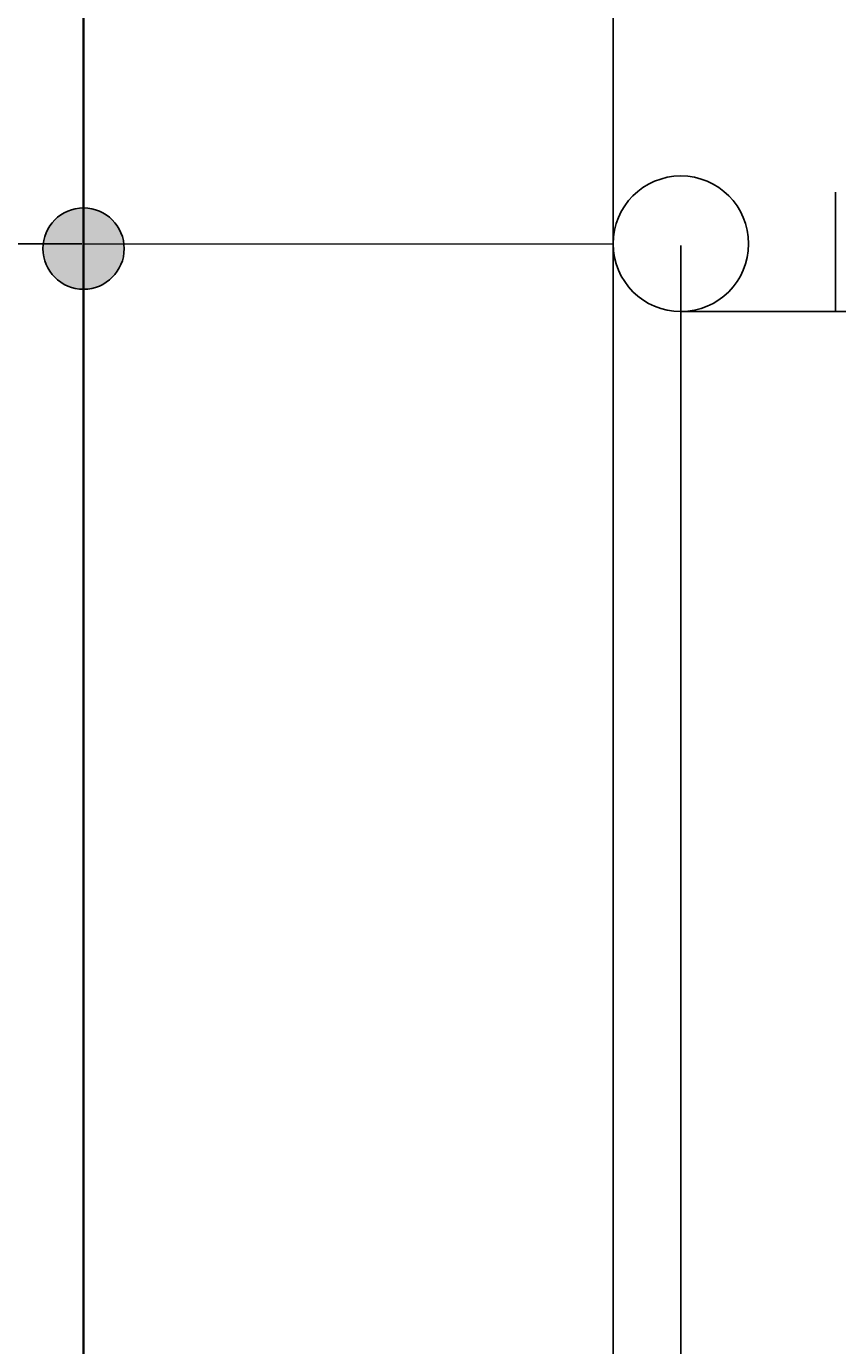
# Model space of a CAD drawing. Units: inches. Extents: x 738 to 1068, y 378 to 757.
# Tile 34 of 41: x 779 to 809, y 606 to 655. Entities that reach past the tile are written whole.
import ezdxf

# ---------------------------------------------------------------- set-up
doc = ezdxf.new("R2010")
doc.units = ezdxf.units.IN
doc.header["$MEASUREMENT"] = 0
for name, color, linetype, lineweight in [('A-ANNO-DIMS', 2, 'Continuous', 18), ('E-CONN', 7, 'Continuous', 25), ('E-CTRL-PBTN', 4, 'Continuous', 25), ('E-CTRL-WIRE', 7, 'Continuous', 18), ('E-POWR-FEED', 7, 'Continuous', 35)]:
    doc.layers.add(name, color=color, linetype=linetype, lineweight=lineweight)
doc.styles.get("Standard").update_dxf_attribs({"font": 'arial.ttf'})
doc.dimstyles.get("Standard").update_dxf_attribs({"dimtxt": 0.18, "dimasz": 0.18, "dimexe": 0.18, "dimexo": 0.0625, "dimgap": 0.09, "dimtad": 0, "dimtih": 1, "dimtoh": 1, "dimdec": 4, "dimzin": 0, "dimdsep": 46, "dimtxsty": 'Standard', "dimcen": 0.09, "dimadec": 0, "dimazin": 0, "dimtfac": 1, "dimtdec": 4, "dimtofl": 0, "dimtmove": 0, "dimatfit": 3, "dimfxl": 1, "dimtolj": 1, "dimtzin": 0, "dimarcsym": 0})

# ---------------------------------------------------------------- blocks, each defined once
blk = doc.blocks.new('RUNG-JUNCTION')
h = blk.add_hatch(color=256)
h.dxf.hatch_style = 1
h.paths.add_polyline_path([(3, 1.5, 1), (0, 1.5, 1)])
blk.add_lwpolyline([(0, 1.5, 1), (3, 1.5, 1)], format="xyb", close=True)
blk = doc.blocks.new('*D23')
at = {"layer": 'A-ANNO-DIMS', "color": 0, "lineweight": -2, "transparency": 16777216}
for p, q in [((781.427, 646.985), (738.194, 646.985)), ((738.374, 646.805), (738.374, 620.214)), ((738.374, 593.26), (738.374, 619.85)), ((781.422, 593.08), (738.194, 593.08))]:
    blk.add_line(p, q, dxfattribs=at)
at = {"layer": 'A-ANNO-DIMS', "color": 0, "transparency": 16777216}
for points in [[(738.344, 646.805), (738.404, 646.805), (738.374, 646.985)], [(738.344, 593.26), (738.404, 593.26), (738.374, 593.08)]]:
    blk.add_solid(points, dxfattribs=at)
at = {"layer": 'Defpoints', "color": 0, "transparency": 16777216}
for p in [(738.374, 646.985), (781.49, 646.985), (781.485, 593.08)]:
    blk.add_point(p, dxfattribs=at)
at = {"layer": 'A-ANNO-DIMS', "color": 0, "transparency": 16777216, "insert": (738.374, 620.032), "char_height": 0.18, "attachment_point": 5}
blk.add_mtext('\\A1;53.91', dxfattribs=at)
blk = doc.blocks.new('*D24')
at = {"layer": 'A-ANNO-DIMS', "color": 0, "lineweight": -2, "transparency": 16777216}
for p, q in [((781.427, 686.329), (738.194, 686.329)), ((738.374, 686.149), (738.374, 666.839)), ((738.374, 647.165), (738.374, 666.475)), ((781.427, 646.985), (738.194, 646.985))]:
    blk.add_line(p, q, dxfattribs=at)
at = {"layer": 'A-ANNO-DIMS', "color": 0, "transparency": 16777216}
for points in [[(738.344, 686.149), (738.404, 686.149), (738.374, 686.329)], [(738.344, 647.165), (738.404, 647.165), (738.374, 646.985)]]:
    blk.add_solid(points, dxfattribs=at)
at = {"layer": 'Defpoints', "color": 0, "transparency": 16777216}
for p in [(738.374, 686.329), (781.49, 686.329), (781.49, 646.985)]:
    blk.add_point(p, dxfattribs=at)
at = {"layer": 'A-ANNO-DIMS', "color": 0, "transparency": 16777216, "insert": (738.374, 666.657), "char_height": 0.18, "attachment_point": 5}
blk.add_mtext('\\A1;39.34', dxfattribs=at)
blk = doc.blocks.new('*D25')
at = {"layer": 'A-ANNO-DIMS', "color": 0, "lineweight": -2, "transparency": 16777216}
for p, q in [((781.49, 646.923), (781.49, 378.239)), ((803.522, 646.923), (803.522, 378.239)), ((781.67, 378.419), (792.111, 378.419)), ((803.342, 378.419), (792.901, 378.419))]:
    blk.add_line(p, q, dxfattribs=at)
at = {"layer": 'A-ANNO-DIMS', "color": 0, "transparency": 16777216}
for points in [[(781.67, 378.449), (781.67, 378.389), (781.49, 378.419)], [(803.342, 378.449), (803.342, 378.389), (803.522, 378.419)]]:
    blk.add_solid(points, dxfattribs=at)
at = {"layer": 'Defpoints', "color": 0, "transparency": 16777216}
for p in [(781.49, 646.985), (803.522, 646.985), (803.522, 378.419)]:
    blk.add_point(p, dxfattribs=at)
at = {"layer": 'A-ANNO-DIMS', "color": 0, "transparency": 16777216, "insert": (792.506, 378.419), "char_height": 0.18, "attachment_point": 5}
blk.add_mtext('\\A1;22.03', dxfattribs=at)
blk = doc.blocks.new('*D31')
at = {"layer": 'A-ANNO-DIMS', "color": 0, "lineweight": -2, "transparency": 16777216}
for p, q in [((781.49, 531.463), (781.49, 756.505)), ((781.67, 756.325), (790.802, 756.325)), ((800.842, 756.325), (791.71, 756.325)), ((801.022, 531.463), (801.022, 756.505))]:
    blk.add_line(p, q, dxfattribs=at)
at = {"layer": 'A-ANNO-DIMS', "color": 0, "transparency": 16777216}
for points in [[(781.67, 756.355), (781.67, 756.295), (781.49, 756.325)], [(800.842, 756.355), (800.842, 756.295), (801.022, 756.325)]]:
    blk.add_solid(points, dxfattribs=at)
at = {"layer": 'Defpoints', "color": 0, "transparency": 16777216}
for p in [(801.022, 756.325), (781.49, 531.401), (801.022, 531.401)]:
    blk.add_point(p, dxfattribs=at)
at = {"layer": 'A-ANNO-DIMS', "color": 0, "transparency": 16777216, "insert": (791.256, 756.325), "char_height": 0.18, "attachment_point": 5}
blk.add_mtext('\\A1;19.532', dxfattribs=at)
blk = doc.blocks.new('*D34')
at = {"layer": 'A-ANNO-DIMS', "color": 0, "lineweight": -2, "transparency": 16777216}
for p, q in [((781.49, 686.266), (781.49, 378.239)), ((830.489, 686.266), (830.489, 378.239)), ((781.67, 378.419), (805.767, 378.419)), ((830.309, 378.419), (806.212, 378.419))]:
    blk.add_line(p, q, dxfattribs=at)
at = {"layer": 'A-ANNO-DIMS', "color": 0, "transparency": 16777216}
for points in [[(781.67, 378.449), (781.67, 378.389), (781.49, 378.419)], [(830.309, 378.449), (830.309, 378.389), (830.489, 378.419)]]:
    blk.add_solid(points, dxfattribs=at)
at = {"layer": 'Defpoints', "color": 0, "transparency": 16777216}
for p in [(781.49, 686.329), (830.489, 686.329), (830.489, 378.419)]:
    blk.add_point(p, dxfattribs=at)
at = {"layer": 'A-ANNO-DIMS', "color": 0, "transparency": 16777216, "insert": (805.99, 378.419), "char_height": 0.18, "attachment_point": 5}
blk.add_mtext('\\A1;49', dxfattribs=at)

msp = doc.modelspace()

# ---------------------------------------------------------------- linework, layer by layer
at = {"layer": 'E-CTRL-PBTN'}
for p, q in [((809.2275, 644.4574), (809.2275, 648.8817)), ((803.5218, 644.4853), (816.0076, 644.4853))]:
    msp.add_line(p, q, dxfattribs=at)
msp.add_lwpolyline([(801.0218, 646.9853, 1), (806.0218, 646.9853, 1)], format="xyb", close=True, dxfattribs=at)
at = {"layer": 'E-CTRL-WIRE'}
msp.add_line((781.4897, 646.9853), (801.0218, 646.9853), dxfattribs=at)
at = {"layer": 'E-POWR-FEED'}
msp.add_line((781.4897, 686.329), (781.4897, 437.7164), dxfattribs=at)

# ---------------------------------------------------------------- block references
at = {"layer": 'E-CONN'}
msp.add_blockref('RUNG-JUNCTION', (779.985, 645.307), dxfattribs=at)

# ---------------------------------------------------------------- dimensions: what is measured, and where the dimension line sits
at = {"layer": 'A-ANNO-DIMS'}
for base, p1, p2, override, picture, middle in [((801.0218, 756.3251), (781.4897, 531.4009), (801.0218, 531.4009), {"dimdec": 3, "dimlfac": 1, "dimrnd": 0, "dimzin": 0, "dimdsep": 46, "dimlunit": 2}, '*D31', (791.2557, 756.3251)), ((830.4893, 378.4191), (781.4897, 686.329), (830.4893, 686.329), {"dimdec": 0, "dimlfac": 1, "dimrnd": 0, "dimzin": 0, "dimdsep": 46, "dimlunit": 2}, '*D34', (805.9895, 378.4191)), ((803.5218, 378.4191), (781.4897, 646.9853), (803.5218, 646.9853), {"dimdec": 2, "dimlfac": 1, "dimrnd": 0, "dimzin": 0, "dimdsep": 46, "dimlunit": 2}, '*D25', (792.5057, 378.4191))]:
    dim = msp.add_linear_dim(base=base, p1=p1, p2=p2, dimstyle='Standard', override=override, dxfattribs=at)
    dim.commit()
    dim.dimension.update_dxf_attribs({"geometry": picture, "text_midpoint": middle})
for base, p1, p2, picture, middle in [((738.3736, 686.329), (781.4897, 646.9853), (781.4897, 686.329), '*D24', (738.3736, 666.6571)), ((738.3736, 646.9853), (781.4846, 593.0796), (781.4897, 646.9853), '*D23', (738.3736, 620.0325))]:
    dim = msp.add_linear_dim(base=base, p1=p1, p2=p2, angle=90, dimstyle='Standard', override={"dimdec": 2, "dimlfac": 1, "dimrnd": 0, "dimzin": 0, "dimdsep": 46, "dimlunit": 2}, dxfattribs=at)
    dim.commit()
    dim.dimension.update_dxf_attribs({"geometry": picture, "text_midpoint": middle})

doc.saveas('drawing.dxf')
